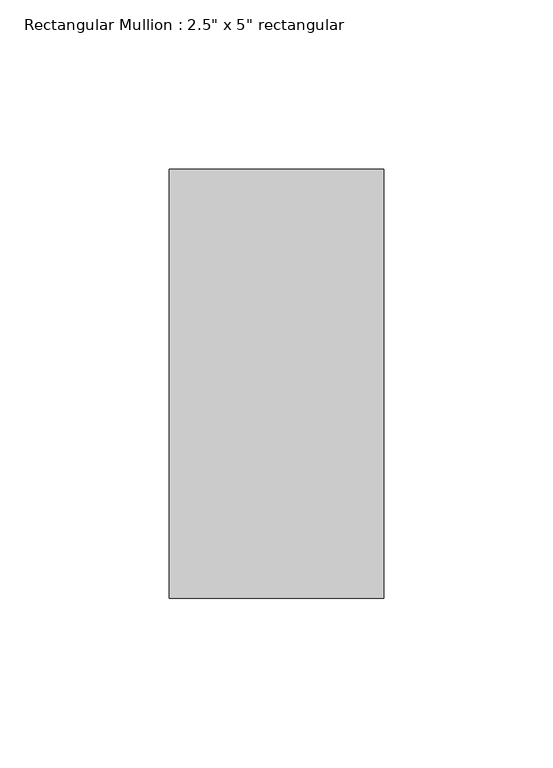
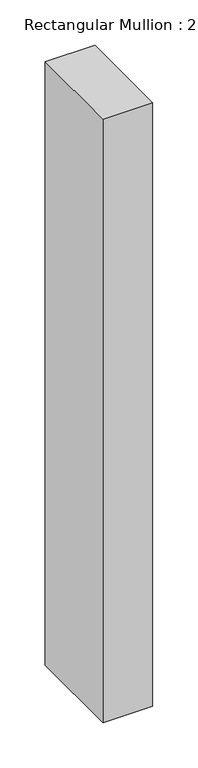
"""IFC4 building model written with IfcOpenShell, lengths in millimetres: member geometry."""

from ifc_helpers import new_model, si_unit, frame, origin, place, context, project, spatial, polyline, outline, extrude, source, transform, mapped, element, save


def member_933cb09f(model_context):
    return source(origin(), model_context, "Body", "SweptSolid", [
        extrude(outline(polyline([(0.0, 63.5), (0.0, -63.5), (-63.5, -63.5), (-63.5, 63.5), (0.0, 63.5)])), frame((0.0, 0.0, -811.2235546), z_axis=(0.0, 0.0, 1.0), x_axis=(1.0, 0.0, 0.0)), (0.0, 0.0, 1.0), 811.2235546),
    ])


if __name__ == "__main__":
    model = new_model("IFC4")
    model_context = context("Model", 3, world=origin())
    ifc_project = project(units=[si_unit("LENGTHUNIT", "METRE", prefix="MILLI")], contexts=[model_context])
    site = spatial("IfcSite", under=ifc_project)
    building = spatial("IfcBuilding", under=site)
    placement = place(None, origin())
    member_shape = member_933cb09f(model_context)
    element("IfcMember", 1, ObjectType="Rectangular Mullion : 2.5\" x 5\" rectangular", at=placement, inside=building, context=model_context, shape_type="MappedRepresentation", body=[
        mapped(member_shape, transform((0.0, 0.0, 0.0), x_axis=(1.0, 0.0, 0.0), y_axis=(0.0, 1.0, 0.0), z_axis=(0.0, 0.0, 1.0))),
    ])
    save(model, "model.ifc")

# Revit data of these elements
# Type "Rectangular Mullion : 2.5\" x 5\" rectangular"
#   built-in parameter 1007304 = 0.416667 (stored number, unit not read)
#   built-in parameter 1007301 = 0.104167 (stored number, unit not read)
#   built-in parameter 1007300 = 0.104167 (stored number, unit not read)
# Element 1 (IfcMember, "Rectangular Mullion : 2.5\" x 5\" rectangular")
#   Materials on its faces: "Aluminum"
# Materials
#   "Aluminum": class "Metal", colour RGB 247 247 247, transparency 0, Description = "Aluminum 6061", Cost = 0
